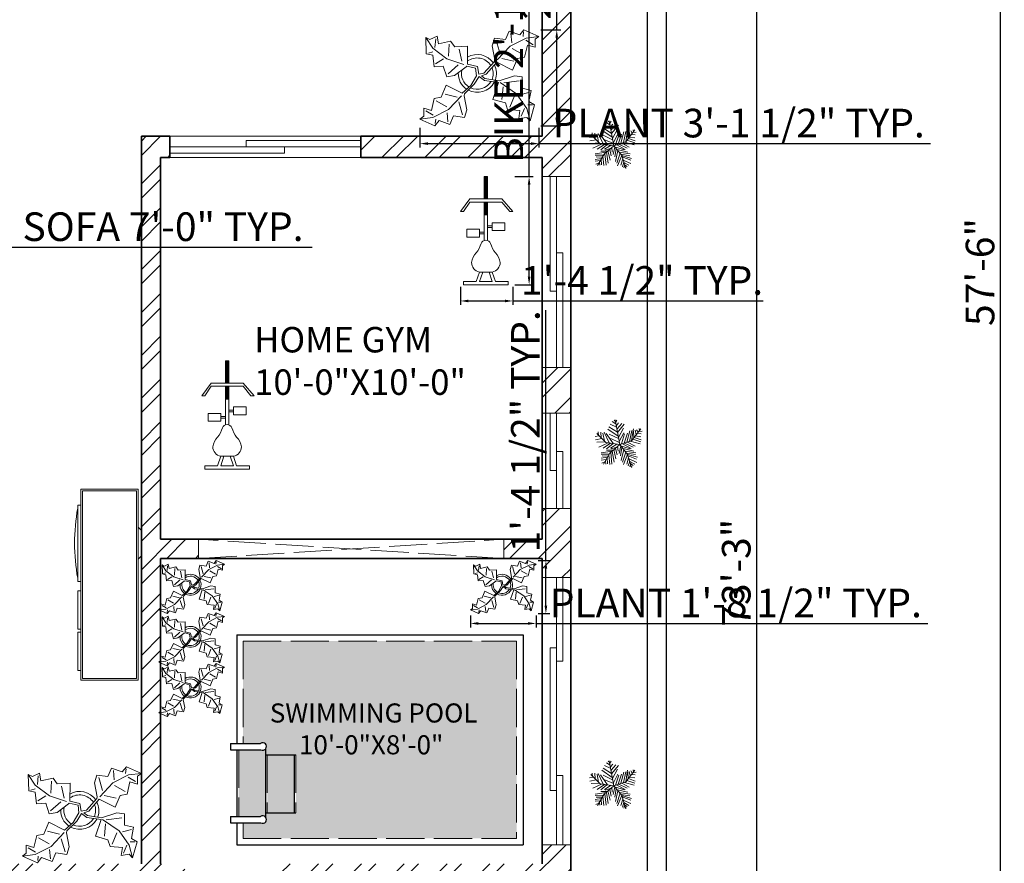
# Model space of a CAD drawing. Units: inches. Extents: x 889 to 1572, y 7262 to 8387.
# Tile 7 of 8: x 1263 to 1572, y 7742 to 8007. Entities that reach past the tile are written whole.
import ezdxf

# ---------------------------------------------------------------- set-up
doc = ezdxf.new("R2010")
doc.units = ezdxf.units.IN
doc.linetypes.add('ACAD_ISO02W100', pattern=[15, 12, -3])
for name, color, linetype, lineweight in [('A-ANNO-DIMS', 2, 'Continuous', 18), ('A-AREA-IDEN', 7, 'Continuous', 18), ('A-EQPM', 8, 'Continuous', 18), ('A-FURN', 8, 'Continuous', 18), ('A-POOL', 4, 'Continuous', 25), ('A-POOL-HIDN', 4, 'ACAD_ISO02W100', 13), ('A-WALL', 7, 'Continuous', 35), ('A-WALL-PATT', 252, 'Continuous', 13), ('C-SITE', 7, 'Continuous', 30), ('L-PLNT', 94, 'Continuous', 13)]:
    doc.layers.add(name, color=color, linetype=linetype, lineweight=lineweight)
for name, color, linetype, lineweight, true_color in [('A-GLAZ', 244, 'Continuous', 18, 0x991b1e), ('A-GLAZ-HIDN', 244, 'ACAD_ISO02W100', 13, 0x991b1e), ('A-POOL-PATT', 152, 'Continuous', 13, 0x2776bb)]:
    doc.layers.add(name, color=color, linetype=linetype, lineweight=lineweight, true_color=true_color)
doc.styles.get("Standard").update_dxf_attribs({"font": 'arial.ttf'})
doc.dimstyles.new('ISO-25', dxfattribs={"dimtxt": 9, "dimasz": 2.5, "dimexe": 1.25, "dimexo": 0.625, "dimtad": 1, "dimlunit": 3, "dimtxsty": 'Standard', "dimcen": 2.5, "dimadec": 0, "dimazin": 0, "dimtfac": 1, "dimtmove": 0, "dimatfit": 3, "dimfxl": 1, "dimarcsym": 0})

# ---------------------------------------------------------------- blocks, each defined once
blk = doc.blocks.new('Entertainment Center')
for p, q in [((-4, 0), (-5, -1)), ((4, 0), (-4, 0)), ((5, -1), (4, 0)), ((-17, -19), (-17, -1)), ((-17, -1), (43, -1)), ((-16.5, -18.5), (-16.5, -1.5)), ((-16.5, -1.5), (42.5, -1.5)), ((42.5, -1.5), (42.5, -18.5)), ((43, -1), (43, -19)), ((42.5, -18.5), (-16.5, -18.5)), ((43, -19), (-17, -19)), ((-12, -20), (-12, -19)), ((12, -20), (-12, -20)), ((12, -19), (12, -20)), ((15, -20), (15, -19)), ((27, -20), (15, -20)), ((27, -19), (27, -20)), ((28, -20), (28, -19)), ((40, -20), (28, -20)), ((40, -19), (40, -20))]:
    blk.add_line(p, q)
blk.add_arc((0, 40), 61, 259.6111, 280.3889)
blk = doc.blocks.new('Plant - Rubber or Philodendron')
for p, q in [((8.8871, 10.7908), (9.9809, 13.4933)), ((9.9809, 13.4933), (13.3837, 12.301)), ((10.5828, 12.6946), (10.8893, 9.7953)), ((13.3837, 12.301), (14.68, 13.9039)), ((14.5816, 13.2037), (14.3848, 11.8033)), ((14.68, 13.9039), (19.3848, 11.8146)), ((-16.2005, 11.4774), (-13.9899, 8.1064)), ((-16.2005, 11.4774), (-14.8639, 10.7964)), ((-16.0159, 6.3329), (-16.2005, 11.4774)), ((-14.8639, 10.7964), (-12.6195, 11.8975)), ((-13.3174, 8.325), (-13.0735, 11.0065)), ((-12.6195, 11.8975), (-12.1909, 9.4345)), ((-12.1909, 9.4345), (-8.3829, 10.3)), ((-8.8369, 9.409), (-9.0894, 5.6095)), ((-8.3829, 10.3), (-7.0549, 8.501)), ((4.6914, 8.8812), (5.3859, 11.2828)), ((5.3859, 11.2828), (8.8871, 10.7908)), ((5.9878, 10.4842), (7.1971, 6.3869)), ((15.3859, 11.3055), (10.3916, 8.7942)), ((15.2875, 10.6053), (17.5907, 9.2105)), ((19.3848, 11.8146), (15.3859, 11.3055)), ((19.3848, 11.8146), (18.1868, 10.9119)), ((18.1868, 10.9119), (18.1925, 8.4119)), ((-14.0069, 5.8704), (-16.0159, 6.3329)), ((-15.3434, 6.5514), (-13.9984, 6.9884)), ((-13.9899, 8.1064), (-9.5434, 4.7185)), ((-7.0549, 8.501), (-3.0284, 8.6941)), ((-4.8529, 4.012), (-5.7184, 7.82)), ((-3.0284, 8.6941), (-3.0709, 3.1041)), ((4.6914, 8.8812), (5.5014, 4.4831)), ((10.3916, 8.7942), (6.2847, 4.4028)), ((14.2977, 6.1031), (10.9934, 7.9956)), ((15.7909, 9.1065), (14.8995, 5.3044)), ((18.1925, 8.4119), (15.7909, 9.1065)), ((-13.5868, 2.2894), (-14.0069, 5.8704)), ((-13.1329, 3.1804), (-10.6614, 4.727)), ((-9.5434, 4.7185), (-4.1917, 2.9888)), ((-3.0709, 3.1041), (0.0797, 2.3163)), ((2.1141, 0.2298), (5.4346, 3.9146)), ((6.1032, 3.6844), (2.8262, -0.031)), ((5.4346, 3.9146), (5.5014, 4.4831)), ((11.1089, 1.1958), (6.1032, 3.6844)), ((7.7005, 4.8881), (11.5025, 3.9967)), ((12.7005, 4.8994), (11.1089, 1.1958)), ((14.8995, 5.3044), (12.7005, 4.8994)), ((-10.6784, 2.491), (-13.5868, 2.2894)), ((-9.5858, -0.8715), (-10.6784, 2.491)), ((-9.1318, 0.0195), (-5.9793, 2.9025)), ((-7.1228, -0.443), (-3.5248, 2.2131)), ((-3.5248, 2.2131), (-3.3011, 2.4355)), ((-3.3011, 2.4355), (-0.5306, 1.7947)), ((-0.5306, 1.7947), (-0.2255, -0.5527)), ((-0.5306, 1.7947), (-0.5306, 1.7947)), ((0.0797, 2.3163), (0.4866, -0.031)), ((0.4866, -0.031), (2.1141, 0.2298)), ((-7.1228, -0.443), (-9.5858, -0.8715)), ((-2.019, -3.6148), (-0.2255, -0.5527)), ((-0.9375, -3.1608), (0.5883, -0.8135)), ((0.5883, -0.8135), (2.2447, -2.0916)), ((2.8262, -0.031), (1.3003, -0.5527)), ((1.3003, -0.5527), (2.4193, -1.4655)), ((2.2447, -2.0916), (6.7108, -2.6626)), ((2.4193, -1.4655), (6.895, -2.1175)), ((4.943, -7.9659), (6.7108, -2.6626)), ((11.6605, -0.5413), (6.895, -2.1175)), ((12.3677, -6.1981), (7.219, -2.6772)), ((8.3544, -2.7453), (13.1973, -2.1704)), ((11.6605, -0.5413), (14.1354, -0.8948)), ((14.1354, -0.8948), (14.1354, -4.4304)), ((-11.3237, -7.2629), (-9.7321, -3.5593)), ((-9.7321, -3.5593), (-4.7264, -6.0479)), ((-2.019, -3.6148), (-4.7264, -6.0479)), ((-4.0579, -6.2781), (-0.9375, -3.1608)), ((8.125, -4.0768), (7.7715, -7.9659)), ((16.2567, -5.8446), (13.4283, -6.5517)), ((14.1354, -4.4304), (16.9638, -5.1375)), ((16.9638, -5.1375), (16.2567, -8.673)), ((-14.4141, -11.4699), (-13.5228, -7.6679)), ((-13.5228, -7.6679), (-11.3237, -7.2629)), ((-12.921, -8.4665), (-9.6166, -10.359)), ((-6.3237, -7.2516), (-10.1257, -6.3602)), ((-9.0148, -11.1577), (-4.9047, -6.8122)), ((-4.611, -12.8477), (-5.8203, -8.7504)), ((-4.1246, -6.8466), (-4.0579, -6.2781)), ((-3.3146, -11.2447), (-4.1246, -6.8466)), ((8.8321, -9.0266), (4.943, -7.9659)), ((9.5392, -11.1479), (8.8321, -9.0266)), ((10.2463, -10.4408), (11.6605, -6.9053)), ((15.5496, -10.7943), (12.3677, -6.1981)), ((16.2567, -8.673), (18.0245, -9.7337)), ((-16.8157, -10.7754), (-14.4141, -11.4699)), ((-16.8101, -13.2754), (-16.8157, -10.7754)), ((-13.9107, -12.9688), (-16.2139, -11.574)), ((-14.0091, -13.669), (-9.0148, -11.1577)), ((-9.206, -15.0581), (-9.5126, -12.1588)), ((-3.3146, -11.2447), (-4.0092, -13.6463)), ((13.4283, -11.5015), (9.5392, -11.1479)), ((13.0748, -13.9763), (13.4283, -11.5015)), ((14.8425, -10.7943), (13.7819, -13.2692)), ((16.6103, -14.6834), (15.5496, -10.7943)), ((17.3174, -9.7337), (15.9032, -9.7337)), ((18.0245, -9.7337), (16.6103, -14.6834)), ((-18.008, -14.1781), (-16.8101, -13.2754)), ((-18.008, -14.1781), (-14.0091, -13.669)), ((-13.3032, -16.2674), (-18.008, -14.1781)), ((-12.0069, -14.6645), (-13.3032, -16.2674)), ((-13.2048, -15.5672), (-13.008, -14.1668)), ((-8.6042, -15.8568), (-12.0069, -14.6645)), ((-7.5103, -13.1543), (-8.6042, -15.8568)), ((-4.0092, -13.6463), (-7.5103, -13.1543)), ((15.5496, -13.6228), (13.0748, -13.9763)), ((16.6103, -14.6834), (15.5496, -13.6228))]:
    blk.add_line(p, q)
for centre, radius, start, end in [((0, 0), 6.1275, 34.37569, 120.1028), ((-0.0601, -0.2075), 5.2461, 33.82192, 124.9414), ((0.0308, 0.1664), 6, 178.6147, 235.1169), ((0.0308, 0.1664), 5, 168.1647, 238.6725), ((-0.2664, 0.1682), 5.2775, 338.4094, 20.03007), ((-0.098, 0.1364), 6.1288, 341.2017, 26.09184), ((-0.0234, 0.3825), 6.1492, 242.5812, 331.2714), ((-0.1102, 0.4886), 5.2883, 247.3711, 327.472)]:
    blk.add_arc(centre, radius, start, end)
blk = doc.blocks.new('Exercise Bike')
for p, q in [((-0.75, 10), (-0.75, 17)), ((-0.75, 17), (0.25, 17)), ((-0.5, 17), (-0.5, 9.9929)), ((-0.25, 10), (-0.25, 17)), ((0, 17), (0, 9.9929)), ((0.25, 17), (0.25, 10)), ((-5.25, 10), (-8.25, 6)), ((-0.75, 10), (-5.25, 10)), ((4.75, 10), (-0.75, 10)), ((8.25, 6), (4.75, 10)), ((-7.25, 6), (-5.25, 9)), ((-5.25, 9), (4.75, 9)), ((-0.75, 5), (-0.75, 9)), ((-0.5, 8.9396), (-0.5, 5)), ((-0.25, 5), (-0.25, 9)), ((0, 8.9396), (0, 5)), ((0.25, 9), (0.25, 5)), ((4.75, 9), (7.25, 6)), ((-8.25, 6), (-7.25, 6)), ((-0.75, -3.0635), (-0.75, 5)), ((-0.75, 5), (0.25, 5)), ((0.25, 5), (0.25, -3.0635)), ((7.25, 6), (8.25, 6)), ((-6.25, -2), (-6.25, 0.5)), ((-2.25, 0.5), (-6.25, 0.5)), ((-2.25, -0.5), (-2.25, 0.5)), ((0.25, 1.5), (1.75, 1.5)), ((0.25, 1), (1.75, 1)), ((1.75, 2.5), (5.75, 2.5)), ((1.75, 1.5), (1.75, 2.5)), ((1.75, 1.5), (1.75, 0)), ((1.75, 0), (5.75, 0)), ((5.75, 2.5), (5.75, 0)), ((-2.25, -2), (-6.25, -2)), ((-2.25, -0.5), (-0.75, -0.5)), ((-2.25, -1), (-2.25, -0.5)), ((-2.25, -1), (-2.25, -2)), ((-0.75, -1), (-2.25, -1)), ((-2.25, -13), (-3.25, -16)), ((-2.25, -16), (-1.25, -13)), ((-2.25, -13), (1.75, -13)), ((0.75, -13), (1.75, -16)), ((1.75, -13), (2.75, -16)), ((-7.25, -16), (-7.25, -17)), ((-4.75, -16), (-7.25, -16)), ((-7.25, -17), (6.75, -17)), ((-3.25, -16), (-4.75, -16)), ((1.75, -16), (-2.25, -16)), ((6.75, -16), (2.75, -16)), ((6.75, -17), (6.75, -16))]:
    blk.add_line(p, q)
for centre, radius, start, end in [((-0.25, -4.625), 1.625, 22.61987, 157.3801), ((-9.6692, -1.9154), 8.1889, 321.6175, 345.2525), ((9.1691, -1.9154), 8.1889, 194.7476, 218.3825), ((0.1685, -10.5843), 4.9531, 133.6443, 173.2256), ((-0.6686, -10.5843), 4.9531, 6.774486, 46.35562), ((-1.7006, -10.0005), 3.0494, 179.9906, 259.6205), ((1.2006, -10.0005), 3.0494, 280.3795, 0.009389)]:
    blk.add_arc(centre, radius, start, end)
blk = doc.blocks.new('*U15')
for p, q in [((-7.288, 39.707), (-21.778, 46.673)), ((-8.737, 47.138), (-17.069, 52.711)), ((-10.186, 53.64), (-13.084, 55.962)), ((0, 0), (-10.5, 57)), ((-9.099, 51.782), (-6.563, 55.962)), ((-7.65, 43.423), (-2.578, 49.46)), ((-5.839, 35.992), (4.667, 48.067)), ((-5.114, 27.632), (10.463, 46.673)), ((-31.5, 4.5), (-52.5, 25.5)), ((-48.585, 21.131), (-49.309, 29.026)), ((-43.513, 28.561), (-42.427, 15.558)), ((-38.442, 26.239), (-34.819, 7.663)), ((-35.544, 28.097), (-24.314, 3.947)), ((-14.533, 2.09), (-30.834, 25.31)), ((-3.665, 19.273), (-27.574, 35.527)), ((-5.114, 28.097), (-24.676, 40.636)), ((-24.314, 23.917), (-2.941, 13.7)), ((-2.941, 16.486), (8.652, 37.85)), ((-1.129, 6.734), (9.014, 26.704)), ((3.942, 1.625), (11.187, 24.381)), ((10.101, 3.483), (17.708, 26.239)), ((16.259, 5.805), (23.142, 31.348)), ((22.055, 7.198), (27.489, 32.277)), ((27, 9), (48, 36)), ((27.127, 9.056), (31.112, 35.992)), ((31.836, 30.883), (32.561, 16.486)), ((35.096, 32.741), (37.27, 22.524)), ((38.719, 34.134), (41.979, 28.561)), ((40.53, 25.775), (48.862, 24.846)), ((43.791, 29.954), (51.036, 30.883)), ((44.153, 36.456), (45.239, 32.741)), ((-47.498, 19.737), (-55.83, 18.344)), ((-40.615, 13.7), (-55.105, 10.913)), ((-33.37, 6.269), (-52.207, 5.34)), ((-28.299, 3.483), (-47.86, -5.805)), ((-21.416, 3.018), (-38.079, -8.128)), ((0, 0), (-31.5, 4.5)), ((-15.982, 2.09), (-30.11, -9.521)), ((0, 0), (-22.5, -19.5)), ((-6.563, 1.161), (-21.416, -8.128)), ((-20.691, 13.7), (-1.129, 4.876)), ((0, 0), (27, 9)), ((0, 0), (18, -22.5)), ((6.478, 1.625), (26.04, -8.592)), ((11.187, 3.483), (30.749, -5.805)), ((18.07, 5.805), (35.096, -3.483)), ((24.229, 7.663), (46.688, 1.625)), ((29.662, 12.307), (48.137, 6.269)), ((33.285, 16.486), (48.862, 10.913)), ((36.183, 19.737), (48.137, 17.88)), ((-17.431, -15.094), (-42.789, -18.809)), ((-24.314, -21.596), (-42.427, -22.06)), ((-22.5, -19.5), (-37.5, -45)), ((-15.257, -12.772), (-30.11, -12.772)), ((-20.691, -18.345), (-17.793, -44.352)), ((-6.563, -5.805), (-19.967, -9.985)), ((-17.069, -15.094), (-12.721, -40.172)), ((-13.446, -11.378), (-8.737, -32.741)), ((-9.461, -8.592), (-6.201, -23.453)), ((-4.752, -3.483), (-3.665, -14.629)), ((2.493, -3.019), (-1.491, -20.202)), ((1.769, -2.555), (24.229, -9.521)), ((5.029, -6.27), (2.131, -25.775)), ((9.014, -11.378), (3.58, -35.992)), ((14.085, -16.951), (6.478, -40.172)), ((7.565, -9.056), (32.198, -14.629)), ((12.274, -15.094), (36.907, -18.809)), ((16.259, -19.738), (36.183, -22.989)), ((18, -22.5), (27, -52.5)), ((-28.299, -29.026), (-42.789, -31.348)), ((-30.834, -34.135), (-42.427, -35.528)), ((-34.457, -39.708), (-40.978, -42.494)), ((-26.849, -26.24), (-40.253, -25.775)), ((-32.646, -36.921), (-31.921, -44.352)), ((-29.023, -30.884), (-27.936, -43.887)), ((-25.038, -23.918), (-22.865, -45.281)), ((18.07, -22.524), (8.289, -45.745)), ((20.244, -30.419), (15.897, -44.816)), ((18.433, -22.524), (40.53, -29.026)), ((19.157, -25.311), (38.719, -33.206)), ((22.78, -37.85), (19.519, -48.532)), ((21.331, -32.741), (39.081, -40.636)), ((22.78, -38.314), (34.372, -44.816)), ((24.591, -43.423), (30.749, -47.603)), ((24.591, -45.745), (23.142, -50.854)), ((26.764, -49.925), (28.213, -50.854))]:
    blk.add_line(p, q)
blk = doc.blocks.new('*D29')
at = {"layer": 'A-ANNO-DIMS', "color": 0, "lineweight": -2, "transparency": 16777216}
for p, q in [((1466.67, 8272.73), (1495.73, 8272.73)), ((1494.48, 8270.23), (1494.48, 7396.23)), ((1466.67, 7393.73), (1495.73, 7393.73))]:
    blk.add_line(p, q, dxfattribs=at)
at = {"layer": 'A-ANNO-DIMS', "color": 0, "transparency": 16777216}
for points in [[(1494.06, 8270.23), (1494.9, 8270.23), (1494.48, 8272.73)], [(1494.06, 7396.23), (1494.9, 7396.23), (1494.48, 7393.73)]]:
    blk.add_solid(points, dxfattribs=at)
at = {"layer": 'Defpoints', "color": 0, "transparency": 16777216}
for p in [(1466.05, 8272.73), (1466.05, 7393.73), (1494.48, 7393.73)]:
    blk.add_point(p, dxfattribs=at)
at = {"layer": 'A-ANNO-DIMS', "color": 0, "transparency": 16777216, "insert": (1489.26, 7833.23), "char_height": 9, "attachment_point": 5, "rotation": 90}
blk.add_mtext('73\'-3"', dxfattribs=at)
blk = doc.blocks.new('GLAZ-SLIDER-60IN')
for p, q in [((0, 60), (0, 24)), ((2, 60), (2, 0)), ((2, 36), (4, 36)), ((4, 36), (4, 0)), ((2, 24), (0, 24))]:
    blk.add_line(p, q)
blk = doc.blocks.new('GLAZ-SLIDER-30IN')
for p, q in [((0, 30), (0, 12)), ((2, 30), (2, 0)), ((4, 18), (2, 18)), ((4, 18), (4, 0)), ((2, 12), (0, 12))]:
    blk.add_line(p, q)
blk = doc.blocks.new('*D47')
at = {"layer": 'A-ANNO-DIMS', "color": 0, "lineweight": -2, "transparency": 16777216}
for p, q in [((1388.66, 7973.07), (1388.66, 7966.84)), ((1426.05, 7973.07), (1426.05, 7966.84)), ((1391.16, 7968.09), (1423.55, 7968.09)), ((1426.05, 7968.09), (1549.2, 7968.09))]:
    blk.add_line(p, q, dxfattribs=at)
at = {"layer": 'A-ANNO-DIMS', "color": 0, "transparency": 16777216}
for points in [[(1391.16, 7968.5), (1391.16, 7967.67), (1388.66, 7968.09)], [(1423.55, 7968.5), (1423.55, 7967.67), (1426.05, 7968.09)]]:
    blk.add_solid(points, dxfattribs=at)
at = {"layer": 'Defpoints', "color": 0, "transparency": 16777216}
for p in [(1388.66, 7973.69), (1426.05, 7973.69), (1426.05, 7968.09)]:
    blk.add_point(p, dxfattribs=at)
at = {"layer": 'A-ANNO-DIMS', "color": 0, "transparency": 16777216, "insert": (1488.87, 7973.37), "char_height": 9, "attachment_point": 5}
blk.add_mtext('PLANT 3\'-1 1/2" TYP.', dxfattribs=at)
blk = doc.blocks.new('*D48')
at = {"layer": 'A-ANNO-DIMS', "color": 0, "lineweight": -2, "transparency": 16777216}
for p, q in [((1431.66, 8003.87), (1431.66, 8062.63)), ((1426.67, 8003.87), (1432.91, 8003.87)), ((1431.66, 7976.19), (1431.66, 8001.37)), ((1426.67, 7973.69), (1432.91, 7973.69))]:
    blk.add_line(p, q, dxfattribs=at)
at = {"layer": 'A-ANNO-DIMS', "color": 0, "transparency": 16777216}
for points in [[(1431.24, 8001.37), (1432.07, 8001.37), (1431.66, 8003.87)], [(1431.24, 7976.19), (1432.07, 7976.19), (1431.66, 7973.69)]]:
    blk.add_solid(points, dxfattribs=at)
at = {"layer": 'Defpoints', "color": 0, "transparency": 16777216}
for p in [(1426.05, 8003.87), (1431.66, 8003.87), (1426.05, 7973.69)]:
    blk.add_point(p, dxfattribs=at)
at = {"layer": 'A-ANNO-DIMS', "color": 0, "transparency": 16777216, "insert": (1426.44, 8034.5), "char_height": 9, "attachment_point": 5, "rotation": 90}
blk.add_mtext('2\'-6" TYP.', dxfattribs=at)
blk = doc.blocks.new('*D49')
at = {"layer": 'A-ANNO-DIMS', "color": 0, "lineweight": -2, "transparency": 16777216}
for p, q in [((1404.49, 7819.76), (1404.49, 7816.03)), ((1406.99, 7817.28), (1422.64, 7817.28)), ((1425.14, 7819.76), (1425.14, 7816.03)), ((1425.14, 7817.28), (1548.29, 7817.28))]:
    blk.add_line(p, q, dxfattribs=at)
at = {"layer": 'A-ANNO-DIMS', "color": 0, "transparency": 16777216}
for points in [[(1406.99, 7817.7), (1406.99, 7816.87), (1404.49, 7817.28)], [(1422.64, 7817.7), (1422.64, 7816.87), (1425.14, 7817.28)]]:
    blk.add_solid(points, dxfattribs=at)
at = {"layer": 'Defpoints', "color": 0, "transparency": 16777216}
for p in [(1404.49, 7820.38), (1425.14, 7820.38), (1425.14, 7817.28)]:
    blk.add_point(p, dxfattribs=at)
at = {"layer": 'A-ANNO-DIMS', "color": 0, "transparency": 16777216, "insert": (1487.97, 7822.56), "char_height": 9, "attachment_point": 5}
blk.add_mtext('PLANT 1\'-8 1/2" TYP.', dxfattribs=at)
blk = doc.blocks.new('*D50')
at = {"layer": 'A-ANNO-DIMS', "color": 0, "lineweight": -2, "transparency": 16777216}
for p, q in [((1428.24, 7837.04), (1428.24, 7915.78)), ((1425.77, 7837.04), (1429.49, 7837.04)), ((1428.24, 7822.88), (1428.24, 7834.54)), ((1425.77, 7820.38), (1429.49, 7820.38))]:
    blk.add_line(p, q, dxfattribs=at)
at = {"layer": 'A-ANNO-DIMS', "color": 0, "transparency": 16777216}
for points in [[(1427.83, 7834.54), (1428.66, 7834.54), (1428.24, 7837.04)], [(1427.83, 7822.88), (1428.66, 7822.88), (1428.24, 7820.38)]]:
    blk.add_solid(points, dxfattribs=at)
at = {"layer": 'Defpoints', "color": 0, "transparency": 16777216}
for p in [(1425.14, 7837.04), (1428.24, 7837.04), (1425.14, 7820.38)]:
    blk.add_point(p, dxfattribs=at)
at = {"layer": 'A-ANNO-DIMS', "color": 0, "transparency": 16777216, "insert": (1422.96, 7877.66), "char_height": 9, "attachment_point": 5, "rotation": 90}
blk.add_mtext('1\'-4 1/2" TYP.', dxfattribs=at)
blk = doc.blocks.new('*D57')
at = {"layer": 'A-ANNO-DIMS', "color": 0, "lineweight": -2, "transparency": 16777216}
for p, q in [((1422.97, 7957.73), (1422.97, 8055.08)), ((1418.49, 7957.73), (1424.22, 7957.73)), ((1422.97, 7926.23), (1422.97, 7955.23)), ((1418.49, 7923.73), (1424.22, 7923.73))]:
    blk.add_line(p, q, dxfattribs=at)
at = {"layer": 'A-ANNO-DIMS', "color": 0, "transparency": 16777216}
for points in [[(1422.55, 7955.23), (1423.38, 7955.23), (1422.97, 7957.73)], [(1422.55, 7926.23), (1423.38, 7926.23), (1422.97, 7923.73)]]:
    blk.add_solid(points, dxfattribs=at)
at = {"layer": 'Defpoints', "color": 0, "transparency": 16777216}
for p in [(1417.87, 7957.73), (1422.97, 7957.73), (1417.87, 7923.73)]:
    blk.add_point(p, dxfattribs=at)
at = {"layer": 'A-ANNO-DIMS', "color": 0, "transparency": 16777216, "insert": (1417.74, 8007.65), "char_height": 9, "attachment_point": 5, "rotation": 90}
blk.add_mtext('BIKE 2\'-10" TYP.', dxfattribs=at)
blk = doc.blocks.new('*D58')
at = {"layer": 'A-ANNO-DIMS', "color": 0, "lineweight": -2, "transparency": 16777216}
for p, q in [((1401.37, 7923.11), (1401.37, 7917.38)), ((1417.87, 7923.11), (1417.87, 7917.38)), ((1403.87, 7918.63), (1415.37, 7918.63)), ((1417.87, 7918.63), (1496.6, 7918.63))]:
    blk.add_line(p, q, dxfattribs=at)
at = {"layer": 'A-ANNO-DIMS', "color": 0, "transparency": 16777216}
for points in [[(1403.87, 7919.05), (1403.87, 7918.21), (1401.37, 7918.63)], [(1415.37, 7919.05), (1415.37, 7918.21), (1417.87, 7918.63)]]:
    blk.add_solid(points, dxfattribs=at)
at = {"layer": 'Defpoints', "color": 0, "transparency": 16777216}
for p in [(1401.37, 7923.73), (1417.87, 7923.73), (1417.87, 7918.63)]:
    blk.add_point(p, dxfattribs=at)
at = {"layer": 'A-ANNO-DIMS', "color": 0, "transparency": 16777216, "insert": (1458.48, 7923.91), "char_height": 9, "attachment_point": 5}
blk.add_mtext('1\'-4 1/2" TYP.', dxfattribs=at)
blk = doc.blocks.new('*D59')
at = {"layer": 'A-ANNO-DIMS', "color": 0, "lineweight": -2, "transparency": 16777216}
for p, q in [((1174.47, 7923.55), (1174.47, 7936.77)), ((1176.97, 7935.52), (1255.97, 7935.52)), ((1258.47, 7923.55), (1258.47, 7936.77)), ((1258.47, 7935.52), (1354.76, 7935.52))]:
    blk.add_line(p, q, dxfattribs=at)
at = {"layer": 'A-ANNO-DIMS', "color": 0, "transparency": 16777216}
for points in [[(1176.97, 7935.94), (1176.97, 7935.11), (1174.47, 7935.52)], [(1255.97, 7935.94), (1255.97, 7935.11), (1258.47, 7935.52)]]:
    blk.add_solid(points, dxfattribs=at)
at = {"layer": 'Defpoints', "color": 0, "transparency": 16777216}
for p in [(1258.47, 7935.52), (1174.47, 7922.92), (1258.47, 7922.92)]:
    blk.add_point(p, dxfattribs=at)
at = {"layer": 'A-ANNO-DIMS', "color": 0, "transparency": 16777216, "insert": (1307.86, 7940.81), "char_height": 9, "attachment_point": 5}
blk.add_mtext('SOFA 7\'-0" TYP.', dxfattribs=at)
blk = doc.blocks.new('*D70')
at = {"layer": 'A-ANNO-DIMS', "color": 0, "lineweight": -2, "transparency": 16777216}
for p, q in [((1436.67, 8272.73), (1572.38, 8272.73)), ((1571.13, 7585.23), (1571.13, 8270.23)), ((1436.67, 7582.73), (1572.38, 7582.73))]:
    blk.add_line(p, q, dxfattribs=at)
at = {"layer": 'A-ANNO-DIMS', "color": 0, "transparency": 16777216}
for points in [[(1570.71, 8270.23), (1571.54, 8270.23), (1571.13, 8272.73)], [(1570.71, 7585.23), (1571.54, 7585.23), (1571.13, 7582.73)]]:
    blk.add_solid(points, dxfattribs=at)
at = {"layer": 'Defpoints', "color": 0, "transparency": 16777216}
for p in [(1436.05, 8272.73), (1571.13, 8272.73), (1436.05, 7582.73)]:
    blk.add_point(p, dxfattribs=at)
at = {"layer": 'A-ANNO-DIMS', "color": 0, "transparency": 16777216, "insert": (1565.91, 7927.73), "char_height": 9, "attachment_point": 5, "rotation": 90}
blk.add_mtext('57\'-6"', dxfattribs=at)
blk = doc.blocks.new('*D74')
at = {"layer": 'A-ANNO-DIMS', "color": 0, "lineweight": -2, "transparency": 16777216}
for p, q in [((1247.05, 8161.11), (1247.05, 7262.35)), ((1253.05, 8161.11), (1253.05, 7262.35)), ((1244.55, 7263.6), (1242.05, 7263.6)), ((1247.05, 7263.6), (1253.05, 7263.6)), ((1255.55, 7263.6), (1283.22, 7263.6))]:
    blk.add_line(p, q, dxfattribs=at)
at = {"layer": 'A-ANNO-DIMS', "color": 0, "transparency": 16777216}
for points in [[(1244.55, 7264.02), (1244.55, 7263.19), (1247.05, 7263.6)], [(1255.55, 7264.02), (1255.55, 7263.19), (1253.05, 7263.6)]]:
    blk.add_solid(points, dxfattribs=at)
at = {"layer": 'Defpoints', "color": 0, "transparency": 16777216}
for p in [(1247.05, 8161.73), (1253.05, 8161.73), (1253.05, 7263.6)]:
    blk.add_point(p, dxfattribs=at)
at = {"layer": 'A-ANNO-DIMS', "color": 0, "transparency": 16777216, "insert": (1270.64, 7268.82), "char_height": 9, "attachment_point": 5}
blk.add_mtext('0\'-6"', dxfattribs=at)

msp = doc.modelspace()

# ---------------------------------------------------------------- hatches: boundary and pattern name
at = {"layer": 'A-POOL-PATT'}
h = msp.add_hatch(color=256, dxfattribs=at)
h.dxf.hatch_style = 1
h.paths.add_polyline_path([(1419.049, 7811.731), (1333.049, 7811.731), (1333.049, 7779.61), (1338.543, 7779.61, -0.9168649), (1340.049, 7777.807), (1340.049, 7776.042), (1349.649, 7776.042), (1349.649, 7757.766), (1340.049, 7757.766), (1340.049, 7756.479, -0.8686135), (1338.651, 7754.61), (1333.049, 7754.61), (1333.049, 7749.731), (1419.049, 7749.731)])
h.paths.add_polyline_path([(1349.049, 7776.042), (1340.649, 7776.042), (1340.649, 7757.766), (1349.049, 7757.766)], flags=17)
h.paths.add_polyline_path([(1340.049, 7777.807, -0.3326058), (1338.651, 7777.61), (1331.649, 7777.61), (1331.649, 7756.61), (1338.543, 7756.61, -0.3627062), (1340.049, 7756.479)])
h.paths.add_polyline_path([(1339.564, 7772.745), (1412.882, 7772.745), (1412.882, 7795.133), (1339.564, 7795.133)], flags=24)
at = {"layer": 'A-WALL-PATT'}
h = msp.add_hatch(dxfattribs=at)
h.set_pattern_fill('ANSI32', color=256)
h.paths.add_polyline_path([(1166.049, 7624.731), (1163.049, 7624.731), (1163.049, 7774.731), (1154.049, 7774.731), (1154.049, 7768.731), (1157.049, 7768.731), (1157.049, 7624.731), (1106.049, 7624.731), (1106.049, 7615.731), (1166.049, 7615.731), (1166.049, 7618.431)])
h.paths.add_polyline_path([(1025.049, 7666.731), (1016.049, 7666.731), (1016.049, 7615.731), (1076.049, 7615.731), (1076.049, 7624.731), (1025.049, 7624.731)])
h.paths.add_polyline_path([(1025.049, 7768.731), (1118.049, 7768.731), (1118.049, 7774.731), (1025.049, 7774.731), (1025.049, 7897.731), (1115.049, 7897.731), (1115.049, 7906.731), (1109.049, 7906.731), (1109.049, 7903.731), (1025.049, 7903.731), (1025.049, 7923.231), (1016.049, 7923.231), (1016.049, 7726.731), (1025.049, 7726.731)])
h.paths.add_polyline_path([(1436.049, 7897.731), (1427.049, 7897.731), (1427.049, 7883.374), (1436.049, 7883.374)])
h.paths.add_polyline_path([(1436.049, 7853.374), (1427.049, 7853.374), (1427.049, 7843.731), (1415.049, 7843.731), (1415.049, 7837.731), (1427.049, 7837.731), (1427.049, 7831.731), (1436.049, 7831.731)])
h.paths.add_polyline_path([(1436.049, 8010.183), (1427.049, 8010.183), (1427.049, 7970.456), (1370.049, 7970.456), (1370.049, 7963.731), (1427.049, 7963.731), (1427.049, 7957.731), (1436.049, 7957.731)])
h.paths.add_polyline_path([(1436.049, 7747.731), (1427.049, 7747.731), (1427.049, 7741.731), (1344.721, 7741.731), (1344.721, 7735.731), (1349.049, 7735.731), (1349.049, 7672.731), (1355.049, 7672.731), (1355.049, 7735.731), (1427.049, 7735.731), (1427.049, 7721.931), (1436.049, 7721.931)])
h.paths.add_polyline_path([(1436.049, 7700.931), (1427.049, 7700.931), (1427.049, 7591.731), (1355.049, 7591.731), (1355.049, 7642.731), (1349.049, 7642.731), (1349.049, 7591.731), (1310.049, 7591.731), (1310.049, 7582.731), (1436.049, 7582.731)])
h.paths.add_polyline_path([(1392.42, 8272.731), (1331.049, 8272.731), (1331.049, 8263.731), (1349.049, 8263.731), (1349.049, 8224.731), (1355.049, 8224.731), (1355.049, 8263.731), (1392.42, 8263.731)])
h.paths.add_polyline_path([(1271.049, 8272.731), (1196.736, 8272.731), (1196.736, 8263.731), (1247.049, 8263.731), (1247.049, 8203.731), (1244.049, 8203.731), (1244.049, 8197.731), (1247.049, 8197.731), (1247.049, 8161.731), (1253.049, 8161.731), (1253.049, 8185.731), (1295.049, 8185.731), (1295.049, 8191.731), (1253.049, 8191.731), (1253.049, 8263.731), (1271.049, 8263.731)])
h.paths.add_polyline_path([(1175.736, 8272.731), (1102.037, 8272.731), (1102.037, 8263.731), (1157.049, 8263.731), (1157.049, 8158.731), (1163.049, 8158.731), (1163.049, 8197.731), (1214.049, 8197.731), (1214.049, 8203.731), (1163.049, 8203.731), (1163.049, 8263.731), (1175.736, 8263.731)])
h.paths.add_polyline_path([(1072.037, 8272.731), (1016.049, 8272.731), (1016.049, 8221.731), (1025.049, 8221.731), (1025.049, 8263.731), (1072.037, 8263.731)])
h.paths.add_polyline_path([(1163.049, 8122.731), (1157.049, 8122.731), (1157.049, 8119.731), (1025.049, 8119.731), (1025.049, 8161.731), (1016.049, 8161.731), (1016.049, 8071.731), (1025.049, 8071.731), (1025.049, 8113.731), (1157.049, 8113.731), (1157.049, 8110.731), (1163.049, 8110.731)])
h.paths.add_polyline_path([(1025.049, 8011.731), (1016.049, 8011.731), (1016.049, 7944.231), (1025.049, 7944.231), (1025.049, 7963.731), (1109.049, 7963.731), (1109.049, 7936.731), (1115.049, 7936.731), (1115.049, 7963.731), (1163.049, 7963.731), (1163.049, 8074.731), (1157.049, 8074.731), (1157.049, 7969.731), (1025.049, 7969.731)])
h.paths.add_polyline_path([(1314.721, 7741.731), (1307.049, 7741.731), (1307.049, 7837.731), (1319.049, 7837.731), (1319.049, 7843.731), (1307.049, 7843.731), (1307.049, 7963.731), (1310.049, 7963.731), (1310.049, 7970.456), (1301.049, 7970.456), (1301.049, 7837.731), (1301.049, 7741.731), (1250.049, 7741.731), (1250.049, 7735.731), (1314.721, 7735.731)])
h.paths.add_polyline_path([(1211.049, 7735.731), (1214.049, 7735.731), (1214.049, 7741.731), (1205.049, 7741.731), (1205.049, 7624.731), (1202.049, 7624.731), (1202.049, 7615.731), (1205.049, 7615.731), (1205.049, 7582.731), (1250.049, 7582.731), (1250.049, 7591.731), (1211.049, 7591.731)])
h.paths.add_polyline_path([(1436.049, 8260.718), (1427.049, 8260.718), (1427.049, 8191.731), (1355.049, 8191.731), (1355.049, 8194.731), (1349.049, 8194.731), (1349.049, 8191.731), (1343.049, 8191.731), (1343.049, 8185.731), (1427.049, 8185.731), (1427.049, 8070.183), (1436.049, 8070.183)])

# ---------------------------------------------------------------- linework, layer by layer
at = {"layer": 'A-GLAZ'}
for p, q in [((1310.049, 7970.456), (1370.049, 7970.456)), ((1310.049, 7963.731), (1370.049, 7963.731)), ((1319.049, 7843.731), (1319.049, 7837.731)), ((1415.049, 7843.731), (1415.049, 7837.731)), ((1431.549, 7831.731), (1431.549, 7747.731)), ((1433.549, 7831.731), (1433.549, 7805.416)), ((1429.549, 7809.579), (1429.549, 7764.767)), ((1431.549, 7809.579), (1429.549, 7809.579)), ((1431.549, 7805.416), (1433.549, 7805.416)), ((1431.549, 7769.534), (1433.549, 7769.534)), ((1433.549, 7769.534), (1433.549, 7747.731)), ((1429.549, 7764.767), (1431.549, 7764.767))]:
    msp.add_line(p, q, dxfattribs=at)
for points in [[(1427.049, 7957.731), (1436.049, 7957.731), (1436.049, 7897.731), (1427.049, 7897.731)], [(1436.049, 7883.374), (1436.049, 7853.374), (1427.049, 7853.374), (1427.049, 7883.374)], [(1427.049, 7831.731), (1436.049, 7831.731), (1436.049, 7747.731), (1427.049, 7747.731)]]:
    msp.add_lwpolyline(points, close=True, dxfattribs=at)
at = {"layer": 'A-GLAZ-HIDN'}
for p, q in [((1319.049, 7837.731), (1415.049, 7843.731)), ((1415.049, 7837.731), (1319.049, 7843.731))]:
    msp.add_line(p, q, dxfattribs=at)
at = {"layer": 'A-POOL'}
for p, q in [((1331.049, 7813.731), (1331.049, 7779.61)), ((1331.049, 7813.731), (1421.049, 7813.731)), ((1421.049, 7813.731), (1421.049, 7747.731)), ((1329.049, 7779.61), (1338.543, 7779.61)), ((1329.049, 7779.61), (1329.049, 7777.61)), ((1329.049, 7777.61), (1338.651, 7777.61)), ((1331.049, 7777.61), (1331.049, 7756.61)), ((1340.049, 7777.807), (1340.049, 7756.479)), ((1340.049, 7776.042), (1349.649, 7776.042)), ((1349.049, 7776.042), (1349.049, 7757.766)), ((1329.049, 7756.61), (1338.543, 7756.61)), ((1329.049, 7756.61), (1329.049, 7754.61)), ((1340.049, 7757.766), (1349.649, 7757.766)), ((1329.049, 7754.61), (1338.651, 7754.61)), ((1331.049, 7754.61), (1331.049, 7747.731)), ((1331.049, 7747.731), (1421.049, 7747.731))]:
    msp.add_line(p, q, dxfattribs=at)
for centre in [(1339.218, 7778.643), (1339.218, 7755.643)]:
    msp.add_arc(centre, 1.179, 241.24911, 124.90528, dxfattribs=at)
at = {"layer": 'A-POOL-HIDN'}
for p, q in [((1333.049, 7811.731), (1419.049, 7811.731)), ((1333.049, 7811.731), (1333.049, 7779.61)), ((1419.049, 7811.731), (1419.049, 7749.731)), ((1331.649, 7777.61), (1331.649, 7756.61)), ((1340.649, 7776.042), (1340.649, 7757.766)), ((1349.649, 7776.042), (1349.649, 7757.766)), ((1333.049, 7754.61), (1333.049, 7749.731)), ((1333.049, 7749.731), (1419.049, 7749.731))]:
    msp.add_line(p, q, dxfattribs=at)
at = {"layer": 'A-WALL'}
for p, q in [((1436.049, 8272.731), (1436.049, 7582.731)), ((1427.049, 8185.731), (1427.049, 7970.456)), ((1301.049, 7970.456), (1310.049, 7970.456)), ((1301.049, 7970.456), (1301.049, 7837.731)), ((1310.049, 7963.731), (1310.049, 7970.456)), ((1370.049, 7963.731), (1370.049, 7970.456)), ((1370.049, 7970.456), (1427.049, 7970.456)), ((1307.049, 7963.731), (1310.049, 7963.731)), ((1307.049, 7963.731), (1307.049, 7843.731)), ((1370.049, 7963.731), (1427.049, 7963.731)), ((1427.049, 7963.731), (1427.049, 7843.731)), ((1307.049, 7843.731), (1427.049, 7843.731)), ((1301.049, 7837.731), (1301.049, 7741.731)), ((1307.049, 7837.731), (1427.049, 7837.731)), ((1307.049, 7837.731), (1307.049, 7741.731)), ((1427.049, 7837.731), (1427.049, 7741.731))]:
    msp.add_line(p, q, dxfattribs=at)
at = {"layer": 'C-SITE'}
for p, q in [((1466.049, 8272.731), (1466.049, 7582.731)), ((1460.049, 8266.729), (1460.049, 7582.731))]:
    msp.add_line(p, q, dxfattribs=at)

# ---------------------------------------------------------------- block references
at = {"layer": 'A-EQPM'}
for p in [(1409.615, 7940.731), (1328.265, 7882.813)]:
    msp.add_blockref('Exercise Bike', p, dxfattribs=at)
at = {"layer": 'A-FURN', "rotation": 270}
msp.add_blockref('Entertainment Center', (1301.049, 7842.505), dxfattribs=at)
at = {"layer": 'A-GLAZ'}
for p, rotation in [((1370.049, 7965.094), 90.00000000000183), ((1433.548, 7957.731), 180)]:
    msp.add_blockref('GLAZ-SLIDER-60IN', p, dxfattribs=dict(at, rotation=rotation))
msp.add_blockref('GLAZ-SLIDER-30IN', (1429.569, 7853.374), dxfattribs=at)
at = {"layer": 'L-PLNT'}
for p in [(1406.664, 7989.962), (1281.664, 7758.36)]:
    msp.add_blockref('Plant - Rubber or Philodendron', p, dxfattribs=at)
for name, p, xscale, yscale, zscale in [('*U15', (1449.619, 7967.434), 0.137481440781912, 0.137481440781912, 0.137481440781912), ('*U15', (1451.461, 7873.492), 0.137481440781912, 0.137481440781912, 0.137481440781912), ('Plant - Rubber or Philodendron', (1316.501, 7829.365), 0.5522845637456728, 0.5522845637456728, 0.5522845637456728), ('Plant - Rubber or Philodendron', (1414.438, 7829.365), 0.5522845637456728, 0.5522845637456728, 0.5522845637456728), ('Plant - Rubber or Philodendron', (1316.501, 7812.979), 0.5522845637456728, 0.5522845637456728, 0.5522845637456728), ('Plant - Rubber or Philodendron', (1316.501, 7797.056), 0.5522845637456728, 0.5522845637456728, 0.5522845637456728), ('*U15', (1449.619, 7766.271), 0.137481440781912, 0.137481440781912, 0.137481440781912)]:
    msp.add_blockref(name, p, dxfattribs=dict(at, xscale=xscale, yscale=yscale, zscale=zscale))

# ---------------------------------------------------------------- texts
at = {"layer": 'A-AREA-IDEN', "attachment_point": 1}
for s, width, insert, char_height in [('HOME GYM\\P10\'-0"X10\'-0"', 62.91344, (1336.515, 7910.457), 8), ('SWIMMING POOL\\P     10\'-0"X8\'-0"', 70.61825, (1341.44, 7792.152), 6)]:
    msp.add_mtext_dynamic_manual_height_columns(s, width=width, gutter_width=12.5, heights=[0], dxfattribs=dict(at, insert=insert, char_height=char_height))

# ---------------------------------------------------------------- dimensions: what is measured, and where the dimension line sits
at = {"layer": 'A-ANNO-DIMS'}
for base, p1, p2, override, picture, middle in [((1571.127, 8272.731), (1436.049, 7582.731), (1436.049, 8272.731), {"dimdec": 1, "dimlfac": 1, "dimrnd": 0, "dimzin": 1, "dimdsep": 46, "dimlunit": 4, "dimfrac": 2}, '*D70', (1565.907, 7927.731)), ((1494.481, 7393.731), (1466.049, 8272.731), (1466.049, 7393.731), {"dimclrd": 0, "dimclre": 0, "dimclrt": 0}, '*D29', (1489.258, 7833.231))]:
    dim = msp.add_linear_dim(base=base, p1=p1, p2=p2, angle=90, dimstyle='ISO-25', override=override, dxfattribs=at)
    dim.commit()
    dim.dimension.update_dxf_attribs({"geometry": picture, "text_midpoint": middle})
dim = msp.add_linear_dim(base=(1253.049, 7263.604), p1=(1247.049, 8161.731), p2=(1253.049, 8161.731), dimstyle='ISO-25', override={"dimdec": 1, "dimlfac": 1, "dimrnd": 0, "dimzin": 1, "dimdsep": 46, "dimlunit": 4, "dimfrac": 2}, dxfattribs=at)
dim.commit()
dim.dimension.update_dxf_attribs({"geometry": '*D74', "text_midpoint": (1270.636, 7268.824)})
for base, p1, p2, text, picture, middle in [((1431.658, 8003.866), (1426.049, 7973.694), (1426.049, 8003.866), '<> TYP.', '*D48', (1426.437, 8034.497)), ((1422.965, 7957.731), (1417.865, 7923.731), (1417.865, 7957.731), 'BIKE <> TYP.', '*D57', (1417.745, 8007.655)), ((1428.242, 7837.043), (1425.144, 7820.38), (1425.144, 7837.043), '<> TYP.', '*D50', (1422.963, 7877.66))]:
    dim = msp.add_linear_dim(base=base, p1=p1, p2=p2, angle=90, text=text, dimstyle='ISO-25', override={"dimdec": 1, "dimlfac": 1, "dimrnd": 0, "dimzin": 1, "dimdsep": 46, "dimlunit": 4, "dimfrac": 2}, dxfattribs=at)
    dim.commit()
    dim.dimension.update_dxf_attribs({"geometry": picture, "text_midpoint": middle})
for base, p1, p2, text, picture, middle in [((1426.049, 7968.085), (1388.656, 7973.694), (1426.049, 7973.694), 'PLANT <> TYP.', '*D47', (1488.874, 7973.367)), ((1258.465, 7935.525), (1174.465, 7922.925), (1258.465, 7922.925), 'SOFA <> TYP.', '*D59', (1307.861, 7940.806)), ((1417.865, 7918.631), (1401.365, 7923.731), (1417.865, 7923.731), '<> TYP.', '*D58', (1458.482, 7923.909)), ((1425.144, 7817.283), (1404.493, 7820.38), (1425.144, 7820.38), 'PLANT <> TYP.', '*D49', (1487.969, 7822.561))]:
    dim = msp.add_linear_dim(base=base, p1=p1, p2=p2, text=text, dimstyle='ISO-25', override={"dimdec": 1, "dimlfac": 1, "dimrnd": 0, "dimzin": 1, "dimdsep": 46, "dimlunit": 4, "dimfrac": 2}, dxfattribs=at)
    dim.commit()
    dim.dimension.update_dxf_attribs({"geometry": picture, "text_midpoint": middle})

doc.saveas('drawing.dxf')
